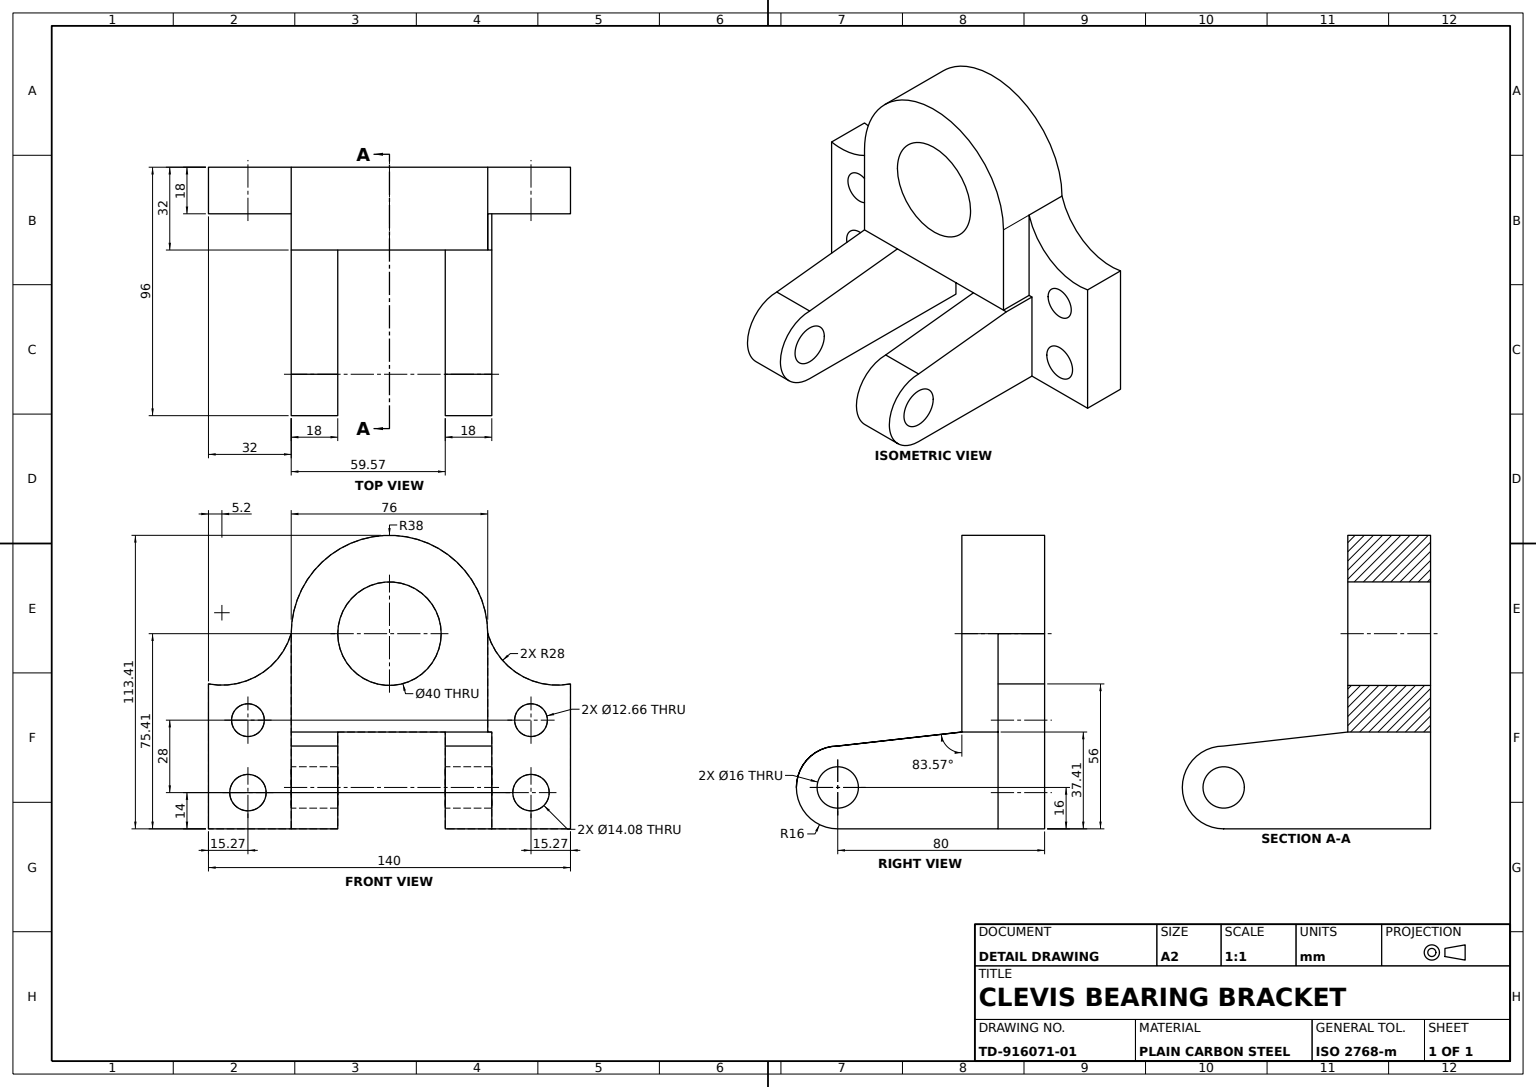
from build123d import *

# Parameters (mm, degrees)
HUB_BODY_PROFILE_R          = 20
HUB_BODY_DEPTH              = 32
MOUNTING_FLANGE_PROFILE_R   = 6.332129474
MOUNTING_FLANGE_PROFILE_R_2 = 7.040095354
MOUNTING_FLANGE_DEPTH       = 18
CLEVIS_ARMS_PROFILE_W       = 18
CLEVIS_ARMS_PROFILE_H       = 37.413354637
CLEVIS_ARMS_DEPTH           = 96
CLEVIS_SLOT_PROFILE_R       = 8
CLEVIS_SLOT_CUT_DEPTH       = 163.994398854


with BuildPart() as part:
    # Hub Body Profile → Hub Body (new body)
    with BuildSketch(Plane.XY):
        with BuildLine():
            Line((38, 0), (38, -38))
            Line((38, -38), (0, -38))
            Line((0, -38), (-38, -38))
            Line((-38, -38), (-38, 0))
            ThreePointArc((-38, 0), (0, 38), (38, 0))
        make_face()
        Circle(HUB_BODY_PROFILE_R, mode=Mode.SUBTRACT)
    extrude(amount=HUB_BODY_DEPTH)

    # Mounting Flange Profile → Mounting Flange (add)
    with BuildSketch(Plane.XY):
        with BuildLine():
            Line((-38, 0), (-38, -75.413354637))
            Line((-38, -75.413354637), (-70, -75.413354637))
            Line((-70, -75.413354637), (-70, -19.413354637))
            ThreePointArc((-70, -19.413354637), (-50.279706144, -15.839023099), (-38, 0))
        make_face()
        with Locations((-54.734551325, -33.413354637)):
            Circle(MOUNTING_FLANGE_PROFILE_R, mode=Mode.SUBTRACT)
        with Locations((-54.734551325, -61.413354637)):
            Circle(MOUNTING_FLANGE_PROFILE_R_2, mode=Mode.SUBTRACT)
    extrude(amount=MOUNTING_FLANGE_DEPTH)

    # Hub Body Mirror: part across plane


with BuildPart() as part_1:
    add(part.part)
    add(part.part.mirror(Plane(origin=(0, 0, 0), x_dir=(0, 0, 1), z_dir=(1, 0, 0))))

    # Clevis Arms Profile → Clevis Arms (add)
    with BuildSketch(Plane.XY):
        with Locations((-29, -56.706677318)):
            Rectangle(CLEVIS_ARMS_PROFILE_W, CLEVIS_ARMS_PROFILE_H)
        with Locations((30.571573125, -56.706677318)):
            Rectangle(CLEVIS_ARMS_PROFILE_W, CLEVIS_ARMS_PROFILE_H)
    extrude(amount=CLEVIS_ARMS_DEPTH)

    # Clevis Slot Profile → Clevis Slot Cut (cut, through all)
    with BuildSketch(Plane.ZY.offset(38)):
        with BuildLine():
            Line((32, -38), (80, -43.413354637))
            ThreePointArc((80, -43.413354637), (91.313708499, -48.099646138), (96, -59.413354637))
            Line((96, -59.413354637), (96, -38))
            Line((96, -38), (32, -38))
        make_face()
        with BuildLine():
            Line((96, -75.413354637), (96, -59.413354637))
            ThreePointArc((96, -59.413354637), (91.313708499, -70.727063136), (80, -75.413354637))
            Line((80, -75.413354637), (96, -75.413354637))
        make_face()
        with Locations((80, -59.413354637)):
            Circle(CLEVIS_SLOT_PROFILE_R)
    extrude(amount=-CLEVIS_SLOT_CUT_DEPTH, mode=Mode.SUBTRACT)


solid = part_1.part
